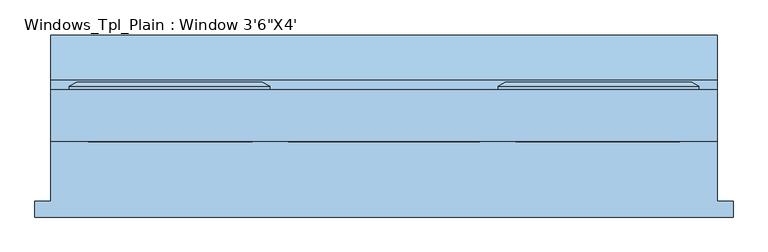
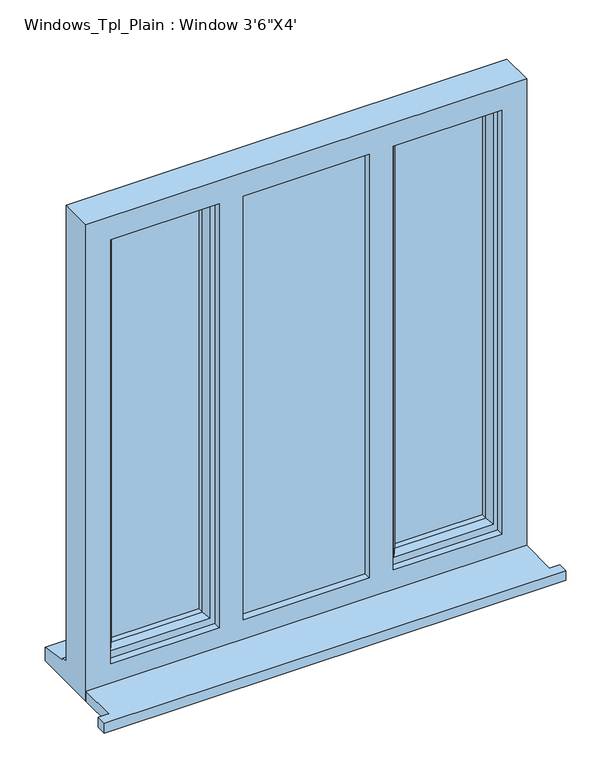
"""IFC4 building model written with IfcOpenShell, lengths in millimetres: window geometry."""

from ifc_helpers import new_model, si_unit, frame, origin, place, context, project, spatial, polyline, outline, extrude, faceted_brep, source, transform, mapped, element, save


def window_63c4cdf6(model_context):
    return source(origin(), model_context, "Body", "SolidModel", [
        extrude(outline(polyline([(-1011.2, -130.8434322), (-1011.2, -105.8434322), (-986.2, -105.8434322), (-986.2, -10.2434322), (80.6, -10.2434322), (80.6, -105.8434322), (105.6, -105.8434322), (105.6, -130.8434322), (-1011.2, -130.8434322)])), frame((0.0, 0.0, 890.8), z_axis=(0.0, 0.0, 1.0), x_axis=(1.0, 0.0, 0.0)), (0.0, 0.0, 1.0), 25.0),
        faceted_brep([(-270.0, 72.7565678, 2080.0), (-270.0, 78.5300705, 2080.0), (-270.0, 78.5300705, 943.8), (-270.0, 72.7565678, 943.8), (-260.0, 7.7565678, 2070.0), (-260.0, 72.7565678, 2070.0), (-260.0, 72.7565678, 953.8), (-260.0, 7.7565678, 953.8), (-220.0, 22.2494677, 2030.0), (-230.1480377, 7.7565678, 2040.1480377), (-230.1480377, 7.7565678, 983.6519623), (-220.0, 22.2494677, 993.8), (-220.0, 36.7565678, 2030.0), (-220.0, 36.7565678, 993.8), (-230.0, 60.7565678, 2040.0), (-230.0, 36.7565678, 2040.0), (-230.0, 36.7565678, 983.8), (-230.0, 60.7565678, 983.8), (-220.0, 78.5300705, 2030.0), (-220.0, 60.7565678, 2030.0), (-220.0, 60.7565678, 993.8), (-220.0, 78.5300705, 993.8), (-237.4457548, 84.3035732, 2047.4457548), (-237.4457548, 84.3035732, 976.3542452), (-259.2153903, 84.3035732, 2069.2153903), (-259.2153903, 84.3035732, 954.5846097), (50.6, 78.5300705, 943.8), (50.6, 72.7565678, 943.8), (40.6, 72.7565678, 953.8), (40.6, 7.7565678, 953.8), (10.7480377, 7.7565678, 983.6519623), (0.6, 22.2494677, 993.8), (0.6, 36.7565678, 993.8), (10.6, 36.7565678, 983.8), (10.6, 60.7565678, 983.8), (0.6, 60.7565678, 993.8), (0.6, 78.5300705, 993.8), (18.0457548, 84.3035732, 976.3542452), (39.8153903, 84.3035732, 954.5846097), (50.6, 78.5300705, 2080.0), (50.6, 72.7565678, 2080.0), (40.6, 72.7565678, 2070.0), (40.6, 7.7565678, 2070.0), (10.7480377, 7.7565678, 2040.1480377), (0.6, 22.2494677, 2030.0), (0.6, 36.7565678, 2030.0), (10.6, 36.7565678, 2040.0), (10.6, 60.7565678, 2040.0), (0.6, 60.7565678, 2030.0), (0.6, 78.5300705, 2030.0), (18.0457548, 84.3035732, 2047.4457548), (39.8153903, 84.3035732, 2069.2153903)], [[[0, 1, 2, 3]], [[4, 5, 6, 7]], [[8, 9, 10, 11]], [[12, 8, 11, 13]], [[14, 15, 16, 17]], [[18, 19, 20, 21]], [[22, 18, 21, 23]], [[1, 24, 25, 2]], [[3, 2, 26, 27]], [[7, 6, 28, 29]], [[11, 10, 30, 31]], [[13, 11, 31, 32]], [[17, 16, 33, 34]], [[21, 20, 35, 36]], [[23, 21, 36, 37]], [[2, 25, 38, 26]], [[27, 26, 39, 40]], [[29, 28, 41, 42]], [[31, 30, 43, 44]], [[32, 31, 44, 45]], [[34, 33, 46, 47]], [[36, 35, 48, 49]], [[37, 36, 49, 50]], [[26, 38, 51, 39]], [[40, 39, 1, 0]], [[3, 27, 40, 0], [5, 41, 28, 6]], [[42, 41, 5, 4]], [[7, 29, 42, 4], [9, 43, 30, 10]], [[44, 43, 9, 8]], [[45, 44, 8, 12]], [[15, 46, 33, 16], [13, 32, 45, 12]], [[47, 46, 15, 14]], [[17, 34, 47, 14], [19, 48, 35, 20]], [[49, 48, 19, 18]], [[50, 49, 18, 22]], [[24, 51, 38, 25], [23, 37, 50, 22]], [[39, 51, 24, 1]]]),
        faceted_brep([(-635.6, 72.7565678, 2080.0), (-635.6, 78.5300705, 2080.0), (-956.2, 78.5300705, 2080.0), (-956.2, 72.7565678, 2080.0), (-645.6, 7.7565678, 2070.0), (-645.6, 72.7565678, 2070.0), (-946.2, 72.7565678, 2070.0), (-946.2, 7.7565678, 2070.0), (-685.6, 22.2494677, 2030.0), (-675.4519623, 7.7565678, 2040.1480377), (-916.3480377, 7.7565678, 2040.1480377), (-906.2, 22.2494677, 2030.0), (-685.6, 36.7565678, 2030.0), (-906.2, 36.7565678, 2030.0), (-675.6, 60.7565678, 2040.0), (-675.6, 36.7565678, 2040.0), (-916.2, 36.7565678, 2040.0), (-916.2, 60.7565678, 2040.0), (-685.6, 78.5300705, 2030.0), (-685.6, 60.7565678, 2030.0), (-906.2, 60.7565678, 2030.0), (-906.2, 78.5300705, 2030.0), (-666.7854344, 84.3035732, 2048.8145656), (-925.0145656, 84.3035732, 2048.8145656), (-647.2307806, 84.3035732, 2068.3692194), (-944.5692194, 84.3035732, 2068.3692194), (-956.2, 78.5300705, 943.8), (-956.2, 72.7565678, 943.8), (-946.2, 72.7565678, 953.8), (-946.2, 7.7565678, 953.8), (-916.3480377, 7.7565678, 983.6519623), (-906.2, 22.2494677, 993.8), (-906.2, 36.7565678, 993.8), (-916.2, 36.7565678, 983.8), (-916.2, 60.7565678, 983.8), (-906.2, 60.7565678, 993.8), (-906.2, 78.5300705, 993.8), (-925.0145656, 84.3035732, 974.9854344), (-944.5692194, 84.3035732, 955.4307806), (-635.6, 78.5300705, 943.8), (-635.6, 72.7565678, 943.8), (-645.6, 72.7565678, 953.8), (-645.6, 7.7565678, 953.8), (-675.4519623, 7.7565678, 983.6519623), (-685.6, 22.2494677, 993.8), (-685.6, 36.7565678, 993.8), (-675.6, 36.7565678, 983.8), (-675.6, 60.7565678, 983.8), (-685.6, 60.7565678, 993.8), (-685.6, 78.5300705, 993.8), (-666.7854344, 84.3035732, 974.9854344), (-647.2307806, 84.3035732, 955.4307806)], [[[0, 1, 2, 3]], [[4, 5, 6, 7]], [[8, 9, 10, 11]], [[12, 8, 11, 13]], [[14, 15, 16, 17]], [[18, 19, 20, 21]], [[22, 18, 21, 23]], [[1, 24, 25, 2]], [[3, 2, 26, 27]], [[7, 6, 28, 29]], [[11, 10, 30, 31]], [[13, 11, 31, 32]], [[17, 16, 33, 34]], [[21, 20, 35, 36]], [[23, 21, 36, 37]], [[2, 25, 38, 26]], [[27, 26, 39, 40]], [[0, 3, 27, 40], [41, 28, 6, 5]], [[29, 28, 41, 42]], [[4, 7, 29, 42], [43, 30, 10, 9]], [[31, 30, 43, 44]], [[32, 31, 44, 45]], [[46, 33, 16, 15], [12, 13, 32, 45]], [[34, 33, 46, 47]], [[14, 17, 34, 47], [48, 35, 20, 19]], [[36, 35, 48, 49]], [[37, 36, 49, 50]], [[51, 38, 25, 24], [22, 23, 37, 50]], [[26, 38, 51, 39]], [[40, 39, 1, 0]], [[42, 41, 5, 4]], [[44, 43, 9, 8]], [[45, 44, 8, 12]], [[47, 46, 15, 14]], [[49, 48, 19, 18]], [[50, 49, 18, 22]], [[39, 51, 24, 1]]]),
        faceted_brep([(80.6, -10.2434322, 2110.0), (-986.2, -10.2434322, 2110.0), (-986.2, -10.2434322, 890.8), (80.6, -10.2434322, 890.8), (20.6, -10.2434322, 2050.0), (20.6, -10.2434322, 965.8), (-242.0, -10.2434322, 965.8), (-242.0, -10.2434322, 2050.0), (-300.0, -10.2434322, 2050.0), (-300.0, -10.2434322, 965.8), (-605.6, -10.2434322, 965.8), (-605.6, -10.2434322, 2050.0), (-663.6, -10.2434322, 2050.0), (-663.6, -10.2434322, 965.8), (-926.2, -10.2434322, 965.8), (-926.2, -10.2434322, 2050.0), (-986.2, 72.7565678, 2110.0), (-986.2, 72.7565678, 941.8), (-986.2, 87.7565678, 940.48767), (-986.2, 87.7565678, 935.5449676), (-986.2, 160.2565678, 924.6088847), (-986.2, 160.2565678, 890.8), (80.6, 72.7565678, 2110.0), (80.6, 72.7565678, 941.8), (-946.2, 72.7565678, 2070.0), (-946.2, 72.7565678, 953.8), (-645.6, 72.7565678, 953.8), (-645.6, 72.7565678, 2070.0), (-605.6, 72.7565678, 2070.0), (-605.6, 72.7565678, 953.8), (-300.0, 72.7565678, 953.8), (-300.0, 72.7565678, 2070.0), (-260.0, 72.7565678, 2070.0), (-260.0, 72.7565678, 953.8), (40.6, 72.7565678, 953.8), (40.6, 72.7565678, 2070.0), (-946.2, 7.7565678, 2070.0), (-946.2, 7.7565678, 953.8), (-615.6, 7.7565678, 2070.0), (-290.0, 7.7565678, 2070.0), (-290.0, 7.7565678, 953.8), (-615.6, 7.7565678, 953.8), (-300.0, 7.7565678, 2050.0), (-605.6, 7.7565678, 2050.0), (-605.6, 7.7565678, 965.8), (-300.0, 7.7565678, 965.8), (-260.0, 7.7565678, 2070.0), (40.6, 7.7565678, 2070.0), (40.6, 7.7565678, 953.8), (-260.0, 7.7565678, 953.8), (20.6, 7.7565678, 2050.0), (-242.0, 7.7565678, 2050.0), (-242.0, 7.7565678, 965.8), (20.6, 7.7565678, 965.8), (-645.6, 7.7565678, 2070.0), (-645.6, 7.7565678, 953.8), (-663.6, 7.7565678, 2050.0), (-926.2, 7.7565678, 2050.0), (-926.2, 7.7565678, 965.8), (-663.6, 7.7565678, 965.8), (-605.6, 31.7565678, 2070.0), (-300.0, 31.7565678, 2070.0), (-290.0, 31.7565678, 2070.0), (-615.6, 31.7565678, 2070.0), (80.6, 160.2565678, 890.8), (80.6, 160.2565678, 924.6088847), (80.6, 87.7565678, 935.5449676), (80.6, 87.7565678, 940.48767), (-605.6, 31.7565678, 953.8), (-615.6, 31.7565678, 953.8), (-290.0, 31.7565678, 953.8), (-300.0, 31.7565678, 953.8)], [[[0, 1, 2, 3], [4, 5, 6, 7], [8, 9, 10, 11], [12, 13, 14, 15]], [[2, 1, 16, 17, 18, 19, 20, 21]], [[17, 16, 22, 23], [24, 25, 26, 27], [28, 29, 30, 31], [32, 33, 34, 35]], [[25, 24, 36, 37]], [[38, 39, 40, 41], [42, 43, 44, 45]], [[46, 47, 48, 49], [50, 51, 52, 53]], [[36, 54, 55, 37], [56, 57, 58, 59]], [[57, 15, 14, 58]], [[1, 0, 22, 16]], [[36, 24, 27, 54]], [[35, 47, 46, 32]], [[60, 28, 31, 61, 62, 39, 38, 63]], [[15, 57, 56, 12]], [[50, 4, 7, 51]], [[11, 43, 42, 8]], [[23, 22, 0, 3, 64, 65, 66, 67]], [[35, 34, 48, 47]], [[4, 50, 53, 5]], [[43, 11, 10, 44]], [[12, 56, 59, 13]], [[27, 26, 55, 54]], [[29, 28, 60, 68]], [[68, 60, 63, 69]], [[69, 63, 38, 41]], [[62, 70, 40, 39]], [[70, 62, 61, 71]], [[71, 61, 31, 30]], [[33, 32, 46, 49]], [[51, 7, 6, 52]], [[8, 42, 45, 9]], [[64, 3, 2, 21]], [[65, 64, 21, 20]], [[66, 65, 20, 19]], [[67, 66, 19, 18]], [[23, 67, 18, 17]], [[26, 25, 37, 55]], [[34, 33, 49, 48]], [[41, 40, 70, 71, 30, 29, 68, 69]], [[6, 5, 53, 52]], [[45, 44, 10, 9]], [[59, 58, 14, 13]]]),
        extrude(outline(polyline([(-675.6, 36.7565678), (-916.2, 36.7565678), (-916.2, 60.7565678), (-675.6, 60.7565678), (-675.6, 36.7565678)])), frame((0.0, 0.0, 983.8), z_axis=(0.0, 0.0, 1.0), x_axis=(1.0, 0.0, 0.0)), (0.0, 0.0, 1.0), 1056.2),
        extrude(outline(polyline([(-615.6, 31.7565678), (-290.0, 31.7565678), (-290.0, 7.7565678), (-615.6, 7.7565678), (-615.6, 31.7565678)])), frame((0.0, 0.0, 953.8), z_axis=(0.0, 0.0, 1.0), x_axis=(1.0, 0.0, 0.0)), (0.0, 0.0, 1.0), 1116.2),
        extrude(outline(polyline([(10.6, 36.7565678), (-230.0, 36.7565678), (-230.0, 60.7565678), (10.6, 60.7565678), (10.6, 36.7565678)])), frame((0.0, 0.0, 983.8), z_axis=(0.0, 0.0, 1.0), x_axis=(1.0, 0.0, 0.0)), (0.0, 0.0, 1.0), 1056.2),
    ])


if __name__ == "__main__":
    model = new_model("IFC4")
    model_context = context("Model", 3, world=origin())
    ifc_project = project(units=[si_unit("LENGTHUNIT", "METRE", prefix="MILLI")], contexts=[model_context])
    site = spatial("IfcSite", under=ifc_project)
    building = spatial("IfcBuilding", under=site)
    placement = place(None, origin())
    window_shape = window_63c4cdf6(model_context)
    element("IfcWindow", 1, ObjectType="Windows_Tpl_Plain : Window 3'6\"X4'", at=placement, inside=building, context=model_context, shape_type="MappedRepresentation", body=[
        mapped(window_shape, transform((0.0, 0.0, 0.0), x_axis=(1.0, 0.0, 0.0), y_axis=(0.0, 1.0, 0.0), z_axis=(0.0, 0.0, 1.0))),
    ])
    save(model, "model.ifc")

# Revit data of these elements
# Type "Windows_Tpl_Plain : Window 3'6\"X4'"
#   Type Mark = "33"
#   Operation = "TriplePanelVertical"
#   Construction Type Id = "GSP4R"
#   Manufacturer = "Revit"
#   Keynote = "L10"
#   Analytic Construction = "1/8 in Pilkington single glazing"
#   Wrap Layers (Ext) from Ext = 0' - 4.03543"
#   Wrap Layers (Int) from Ext = 0' - 6.98819"
#   Window Board Projection = 0' - 0.98425"
#   Window Board Extension = 0' - 0.98425"
#   Visual Light Transmittance = 0.9
#   Solar Heat Gain Coefficient = 0.78
#   Rough Width = 3' - 6"
#   Rough Height = 4' - 0"
#   Height = 4' - 0"
#   Width = 3' - 6"
#   Heat Transfer Coefficient (U) = 0.6496 BTU/(h·ft²·°F)
#   Glazing Thickness = 0' - 0.94488"
#   FrameOffset - External = 0' - 1.9685"
#   Frame Depth = 0' - 2.55906"
#   Default Head Height = 6' - 11.07087"
#   Cill Depth = 0' - 3.44488"
#   Cavity Closer Width = 0' - 1.9685"
#   Cavity Closer Offset from Ext = 0' - 4.03543"
#   Cavity Closer Depth = 0' - 3.34646"
#   Vis - Cavity Closers = yes
#   Define Thermal Properties by = 1
#   Material Trim = Window Frame
#   Material Glass = Glass
#   Material Frame = Window Frame
#   Wall Closure = (empty or 0)
# Element 1 (IfcWindow, "Windows_Tpl_Plain : Window 3'6\"X4'")
#   Materials on its faces: "Window Frame", "Glass"
# Materials
#   "Window Frame": colour RGB 249 249 249, transparency 0
#   "Glass": class "Glass", colour RGB 0 128 192, transparency 0.75, Description = "Soda Lime Glass", Cost = 0
